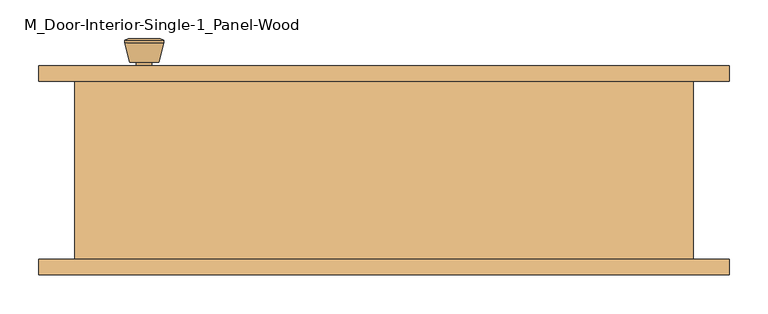
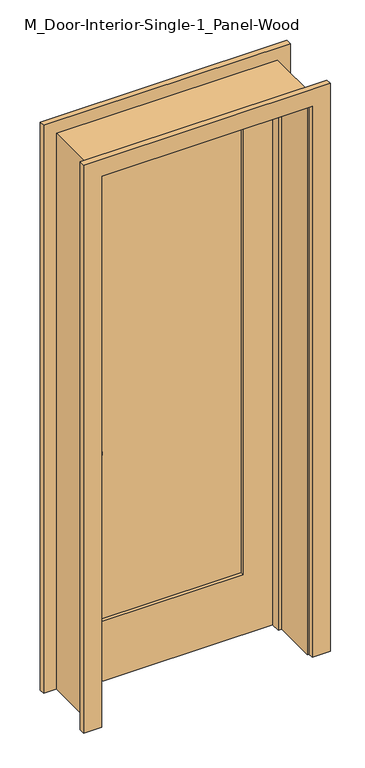
"""IFC4 building model written with IfcOpenShell, lengths in millimetres: door geometry, M_Door-Interior-Single-1_Panel-Wood."""

from ifc_helpers import new_model, si_unit, point, frame, frame_2d, origin, place, context, project, spatial, polyline, circle_curve, trimmed, segment, composite_curve, outline, extrude, faceted_brep, source, transform, mapped, element, save
from ifc_brep_helpers import plane_surface, cylinder_surface, revolved_surface, advanced_brep


def m_door_interior_single_1_panel_wood_d9b71ff8(model_context):
    return source(origin(), model_context, "Body", "SolidModel", [
        advanced_brep(
        [(-310.0, 70.825, 914.4), (-300.0, 70.825, 914.4), (-320.0, 70.825, 914.4), (-289.5241324, 21.825, 914.4), (-310.0, 21.825, 914.4), (-330.4758676, 21.825, 914.4), (-285.0, 23.6528681, 914.4), (-335.0, 23.6528681, 914.4), (-285.0, 27.1165463, 914.4), (-335.0, 27.1165463, 914.4), (-291.363764, 51.825, 914.4), (-328.636236, 51.825, 914.4), (-300.0, 51.825, 914.4), (-320.0, 51.825, 914.4)],
        [
            (0, 1),
            (1, 2, circle_curve(frame((-310.0, 70.825, 914.4), z_axis=(0.0, 1.0, 0.0), x_axis=(-1.0, 0.0, 0.0)), 10.0)),
            (2, 0),
            (2, 1, circle_curve(frame((-310.0, 70.825, 914.4), z_axis=(0.0, 1.0, 0.0), x_axis=(-1.0, 0.0, 0.0)), 10.0)),
            (3, 4),
            (4, 5),
            (5, 3, circle_curve(frame((-310.0, 21.825, 914.4), z_axis=(0.0, -1.0, 0.0), x_axis=(-1.0, 0.0, 0.0)), 20.4758676)),
            (3, 5, circle_curve(frame((-310.0, 21.825, 914.4), z_axis=(0.0, -1.0, 0.0), x_axis=(-1.0, 0.0, 0.0)), 20.4758676)),
            (6, 3),
            (5, 7),
            (7, 6, circle_curve(frame((-310.0, 23.6528681, 914.4), z_axis=(0.0, -1.0, 0.0), x_axis=(-1.0, 0.0, 0.0)), 25.0)),
            (6, 7, circle_curve(frame((-310.0, 23.6528681, 914.4), z_axis=(0.0, -1.0, 0.0), x_axis=(-1.0, 0.0, 0.0)), 25.0)),
            (8, 6),
            (7, 9),
            (9, 8, circle_curve(frame((-310.0, 27.1165463, 914.4), z_axis=(0.0, -1.0, 0.0), x_axis=(-1.0, 0.0, 0.0)), 25.0)),
            (8, 9, circle_curve(frame((-310.0, 27.1165463, 914.4), z_axis=(0.0, -1.0, 0.0), x_axis=(-1.0, 0.0, 0.0)), 25.0)),
            (10, 8),
            (9, 11),
            (11, 10, circle_curve(frame((-310.0, 51.825, 914.4), z_axis=(0.0, -1.0, 0.0), x_axis=(-1.0, 0.0, 0.0)), 18.636236)),
            (10, 11, circle_curve(frame((-310.0, 51.825, 914.4), z_axis=(0.0, -1.0, 0.0), x_axis=(-1.0, 0.0, 0.0)), 18.636236)),
            (12, 10),
            (11, 13),
            (13, 12, circle_curve(frame((-310.0, 51.825, 914.4), z_axis=(0.0, -1.0, 0.0), x_axis=(-1.0, 0.0, 0.0)), 10.0)),
            (12, 13, circle_curve(frame((-310.0, 51.825, 914.4), z_axis=(0.0, -1.0, 0.0), x_axis=(-1.0, 0.0, 0.0)), 10.0)),
            (1, 12),
            (13, 2),
        ],
        [
            plane_surface(frame((-310.0, 70.825, 914.4), z_axis=(0.0, 1.0, 0.0), x_axis=(-1.0, 0.0, 0.0))),
            plane_surface(frame((-310.0, 21.825, 914.4), z_axis=(0.0, -1.0, 0.0), x_axis=(-1.0, 0.0, 0.0))),
            revolved_surface(polyline([(-330.4758676, 21.825, 914.4), (-335.0, 23.6528681, 914.4)]), (-310.0, 70.825, 914.4), (0.0, 1.0, 0.0)),
            cylinder_surface(frame((-310.0, 70.825, 914.4), z_axis=(0.0, 1.0, 0.0), x_axis=(-1.0, 0.0, 0.0)), 25.0),
            revolved_surface(polyline([(-335.0, 27.1165463, 914.4), (-328.636236, 51.825, 914.4)]), (-310.0, 70.825, 914.4), (0.0, 1.0, 0.0)),
            plane_surface(frame((-310.0, 51.825, 914.4), z_axis=(0.0, 1.0, 0.0), x_axis=(-1.0, 0.0, 0.0))),
            cylinder_surface(frame((-310.0, 70.825, 914.4), z_axis=(0.0, 1.0, 0.0), x_axis=(-1.0, 0.0, 0.0)), 10.0),
        ],
        [
            (0, [[1, 2, 3]]),
            (0, [[-3, 4, -1]]),
            (1, [[5, 6, 7]]),
            (1, [[-6, -5, 8]]),
            (2, [[9, -7, 10, 11]]),
            (2, [[-10, -8, -9, 12]]),
            (3, [[13, -11, 14, 15]]),
            (3, [[-14, -12, -13, 16]]),
            (4, [[17, -15, 18, 19]]),
            (4, [[-18, -16, -17, 20]]),
            (5, [[21, -19, 22, 23]]),
            (5, [[-22, -20, -21, 24]]),
            (6, [[25, -23, 26, -2]]),
            (6, [[-26, -24, -25, -4]]),
        ],
    ),
        extrude(outline(composite_curve([segment(trimmed(circle_curve(frame_2d((914.4, -310.0)), 30.0), [point((914.4, -340.0))], [point((914.4, -280.0))], False, "CARTESIAN"), True, "CONTINUOUS"), segment(trimmed(circle_curve(frame_2d((914.4, -310.0)), 30.0), [point((914.4, -280.0))], [point((914.4, -340.0))], False, "CARTESIAN"), True, "CONTINUOUS")], self_intersect=False)), frame((0.0, 70.825, 0.0), z_axis=(0.0, 1.0, 0.0), x_axis=(0.0, 0.0, 1.0)), (0.0, 0.0, 1.0), 6.0),
        advanced_brep(
        [(-310.0, 117.825, 914.4), (-320.0, 117.825, 914.4), (-300.0, 117.825, 914.4), (-289.5241324, 166.825, 914.4), (-330.4758676, 166.825, 914.4), (-310.0, 166.825, 914.4), (-285.0, 164.9971319, 914.4), (-335.0, 164.9971319, 914.4), (-285.0, 161.5334537, 914.4), (-335.0, 161.5334537, 914.4), (-291.363764, 136.825, 914.4), (-328.636236, 136.825, 914.4), (-300.0, 136.825, 914.4), (-320.0, 136.825, 914.4)],
        [
            (0, 1),
            (1, 2, circle_curve(frame((-310.0, 117.825, 914.4), z_axis=(0.0, -1.0, 0.0), x_axis=(-1.0, 0.0, 0.0)), 10.0)),
            (2, 0),
            (2, 1, circle_curve(frame((-310.0, 117.825, 914.4), z_axis=(0.0, -1.0, 0.0), x_axis=(-1.0, 0.0, 0.0)), 10.0)),
            (3, 4, circle_curve(frame((-310.0, 166.825, 914.4), z_axis=(0.0, 1.0, 0.0), x_axis=(-1.0, 0.0, 0.0)), 20.4758676)),
            (4, 5),
            (5, 3),
            (4, 3, circle_curve(frame((-310.0, 166.825, 914.4), z_axis=(0.0, 1.0, 0.0), x_axis=(-1.0, 0.0, 0.0)), 20.4758676)),
            (6, 7, circle_curve(frame((-310.0, 164.9971319, 914.4), z_axis=(0.0, 1.0, 0.0), x_axis=(-1.0, 0.0, 0.0)), 25.0)),
            (7, 4),
            (3, 6),
            (7, 6, circle_curve(frame((-310.0, 164.9971319, 914.4), z_axis=(0.0, 1.0, 0.0), x_axis=(-1.0, 0.0, 0.0)), 25.0)),
            (8, 9, circle_curve(frame((-310.0, 161.5334537, 914.4), z_axis=(0.0, 1.0, 0.0), x_axis=(-1.0, 0.0, 0.0)), 25.0)),
            (9, 7),
            (6, 8),
            (9, 8, circle_curve(frame((-310.0, 161.5334537, 914.4), z_axis=(0.0, 1.0, 0.0), x_axis=(-1.0, 0.0, 0.0)), 25.0)),
            (10, 11, circle_curve(frame((-310.0, 136.825, 914.4), z_axis=(0.0, 1.0, 0.0), x_axis=(-1.0, 0.0, 0.0)), 18.636236)),
            (11, 9),
            (8, 10),
            (11, 10, circle_curve(frame((-310.0, 136.825, 914.4), z_axis=(0.0, 1.0, 0.0), x_axis=(-1.0, 0.0, 0.0)), 18.636236)),
            (12, 13, circle_curve(frame((-310.0, 136.825, 914.4), z_axis=(0.0, 1.0, 0.0), x_axis=(-1.0, 0.0, 0.0)), 10.0)),
            (13, 11),
            (10, 12),
            (13, 12, circle_curve(frame((-310.0, 136.825, 914.4), z_axis=(0.0, 1.0, 0.0), x_axis=(-1.0, 0.0, 0.0)), 10.0)),
            (1, 13),
            (12, 2),
        ],
        [
            plane_surface(frame((-310.0, 117.825, 914.4), z_axis=(0.0, -1.0, 0.0), x_axis=(-1.0, 0.0, 0.0))),
            plane_surface(frame((-310.0, 166.825, 914.4), z_axis=(0.0, 1.0, 0.0), x_axis=(-1.0, 0.0, 0.0))),
            revolved_surface(polyline([(-330.4758676, 166.825, 914.4), (-335.0, 164.9971319, 914.4)]), (-310.0, 117.825, 914.4), (0.0, -1.0, 0.0)),
            cylinder_surface(frame((-310.0, 117.825, 914.4), z_axis=(0.0, -1.0, 0.0), x_axis=(-1.0, 0.0, 0.0)), 25.0),
            revolved_surface(polyline([(-335.0, 161.5334537, 914.4), (-328.636236, 136.825, 914.4)]), (-310.0, 117.825, 914.4), (0.0, -1.0, 0.0)),
            plane_surface(frame((-310.0, 136.825, 914.4), z_axis=(0.0, -1.0, 0.0), x_axis=(-1.0, 0.0, 0.0))),
            cylinder_surface(frame((-310.0, 117.825, 914.4), z_axis=(0.0, -1.0, 0.0), x_axis=(-1.0, 0.0, 0.0)), 10.0),
        ],
        [
            (0, [[1, 2, 3]]),
            (0, [[-3, 4, -1]]),
            (1, [[5, 6, 7]]),
            (1, [[8, -7, -6]]),
            (2, [[9, 10, -5, 11]]),
            (2, [[12, -11, -8, -10]]),
            (3, [[13, 14, -9, 15]]),
            (3, [[16, -15, -12, -14]]),
            (4, [[17, 18, -13, 19]]),
            (4, [[20, -19, -16, -18]]),
            (5, [[21, 22, -17, 23]]),
            (5, [[24, -23, -20, -22]]),
            (6, [[-2, 25, -21, 26]]),
            (6, [[-4, -26, -24, -25]]),
        ],
    ),
        extrude(outline(composite_curve([segment(trimmed(circle_curve(frame_2d((914.4, -310.0)), 30.0), [point((914.4, -340.0))], [point((914.4, -280.0))], False, "CARTESIAN"), True, "CONTINUOUS"), segment(trimmed(circle_curve(frame_2d((914.4, -310.0)), 30.0), [point((914.4, -280.0))], [point((914.4, -340.0))], False, "CARTESIAN"), True, "CONTINUOUS")], self_intersect=False)), frame((0.0, 111.825, 0.0), z_axis=(0.0, 1.0, 0.0), x_axis=(0.0, 0.0, 1.0)), (0.0, 0.0, 1.0), 6.0),
        faceted_brep([(400.0, 111.825, 0.0), (400.0, -118.175, 0.0), (375.0, -118.175, 0.0), (375.0, 41.9, 0.0), (362.3, 41.9, 0.0), (362.3, 76.825, 0.0), (375.0, 76.825, 0.0), (375.0, 111.825, 0.0), (400.0, 111.825, 2125.0), (400.0, -118.175, 2125.0), (-400.0, -118.175, 2125.0), (-400.0, -118.175, 0.0), (-375.0, -118.175, 0.0), (-375.0, -118.175, 2100.0), (375.0, -118.175, 2100.0), (375.0, 41.9, 2100.0), (-375.0, 41.9, 2100.0), (-375.0, 41.9, 0.0), (-362.3, 41.9, 0.0), (-362.3, 41.9, 2087.3), (362.3, 41.9, 2087.3), (362.3, 76.825, 2087.3), (-362.3, 76.825, 2087.3), (-362.3, 76.825, 0.0), (-375.0, 76.825, 0.0), (-375.0, 76.825, 2100.0), (375.0, 76.825, 2100.0), (375.0, 111.825, 2100.0), (-375.0, 111.825, 2100.0), (-375.0, 111.825, 0.0), (-400.0, 111.825, 0.0), (-400.0, 111.825, 2125.0)], [[[0, 1, 2, 3, 4, 5, 6, 7]], [[1, 0, 8, 9]], [[2, 1, 9, 10, 11, 12, 13, 14]], [[3, 2, 14, 15]], [[4, 3, 15, 16, 17, 18, 19, 20]], [[5, 4, 20, 21]], [[6, 5, 21, 22, 23, 24, 25, 26]], [[7, 6, 26, 27]], [[0, 7, 27, 28, 29, 30, 31, 8]], [[9, 8, 31, 10]], [[15, 14, 13, 16]], [[21, 20, 19, 22]], [[27, 26, 25, 28]], [[30, 29, 24, 23, 18, 17, 12, 11]], [[10, 31, 30, 11]], [[16, 13, 12, 17]], [[22, 19, 18, 23]], [[28, 25, 24, 29]]]),
        extrude(outline(polyline([(2100.0, -375.0), (0.0, -375.0), (0.0, 375.0), (2100.0, 375.0), (2100.0, -375.0)]), holes=[polyline([(1980.0, -255.0), (1980.0, 255.0), (230.0, 255.0), (230.0, -255.0), (1980.0, -255.0)])]), frame((0.0, 76.825, 0.0), z_axis=(0.0, 1.0, 0.0), x_axis=(0.0, 0.0, 1.0)), (0.0, 0.0, 1.0), 35.0),
        extrude(outline(polyline([(255.0, 88.4916667), (-255.0, 88.4916667), (-255.0, 100.1583333), (255.0, 100.1583333), (255.0, 88.4916667)])), frame((0.0, 0.0, 230.0), z_axis=(0.0, 0.0, 1.0), x_axis=(1.0, 0.0, 0.0)), (0.0, 0.0, 1.0), 1750.0),
        extrude(outline(polyline([(0.0, 381.35), (0.0, 446.35), (2171.35, 446.35), (2171.35, -446.35), (0.0, -446.35), (0.0, -381.35), (2106.35, -381.35), (2106.35, 381.35), (0.0, 381.35)])), frame((0.0, 111.825, 0.0), z_axis=(0.0, 1.0, 0.0), x_axis=(0.0, 0.0, 1.0)), (0.0, 0.0, 1.0), 20.0),
        extrude(outline(polyline([(0.0, 381.35), (0.0, 446.35), (2171.35, 446.35), (2171.35, -446.35), (0.0, -446.35), (0.0, -381.35), (2106.35, -381.35), (2106.35, 381.35), (0.0, 381.35)])), frame((0.0, -138.175, 0.0), z_axis=(0.0, 1.0, 0.0), x_axis=(0.0, 0.0, 1.0)), (0.0, 0.0, 1.0), 20.0),
    ])


if __name__ == "__main__":
    model = new_model("IFC4")
    model_context = context("Model", 3, world=origin())
    ifc_project = project(units=[si_unit("LENGTHUNIT", "METRE", prefix="MILLI")], contexts=[model_context])
    site = spatial("IfcSite", under=ifc_project)
    building = spatial("IfcBuilding", under=site)
    placement = place(None, origin())
    m_door_interior_single_1_panel_wood_shape = m_door_interior_single_1_panel_wood_d9b71ff8(model_context)
    element("IfcDoor", 1, ObjectType="M_Door-Interior-Single-1_Panel-Wood", at=placement, inside=building, context=model_context, shape_type="MappedRepresentation", body=[
        mapped(m_door_interior_single_1_panel_wood_shape, transform((0.0, 0.0, 0.0), x_axis=(1.0, 0.0, 0.0), y_axis=(0.0, 1.0, 0.0), z_axis=(0.0, 0.0, 1.0))),
    ])
    save(model, "model.ifc")

# Revit data of these elements
# Type "M_Door-Interior-Single-1_Panel-Wood"
#   Type Mark = "23"
#   Assembly Code = "C1020300"
#   Analytic Construction = "Wooden"
#   Top Rail = 120 mm
#   Thickness = 35 mm
#   Thermal Resistance (R) = 0.455703 (m²·K)/W
#   Swing Angle [instance default] = 90.00°
#   Stiles = 120 mm
#   Rough Width = 800 mm
#   Rough Height = 2125 mm
#   Height = 2100 mm
#   Width = 750 mm
#   Heat Transfer Coefficient (U) = 2.19465 W/(m²·K)
#   Bottom Rail = 230 mm
#   Trim Material = Cherry
#   Panel Material = Cherry
#   Frame Material = Cherry
#   Door Handle Material = Aluminum
#   Visual Light Transmittance = 0
#   Solar Heat Gain Coefficient = 0
#   Wall Closure = (empty or 0)
#   Function = (empty or 0)
# Element 1 (IfcDoor, "M_Door-Interior-Single-1_Panel-Wood")
#   Materials on its faces: "Cherry", "Aluminum"
# Materials
#   "Cherry": class "Wood", colour RGB 154 107 61, transparency 0, Description = "Prunus Serotina", Cost = 0
#   "Aluminum": class "Metal", colour RGB 244 244 244, transparency 0, Description = "Aluminum 6061", Cost = 0
